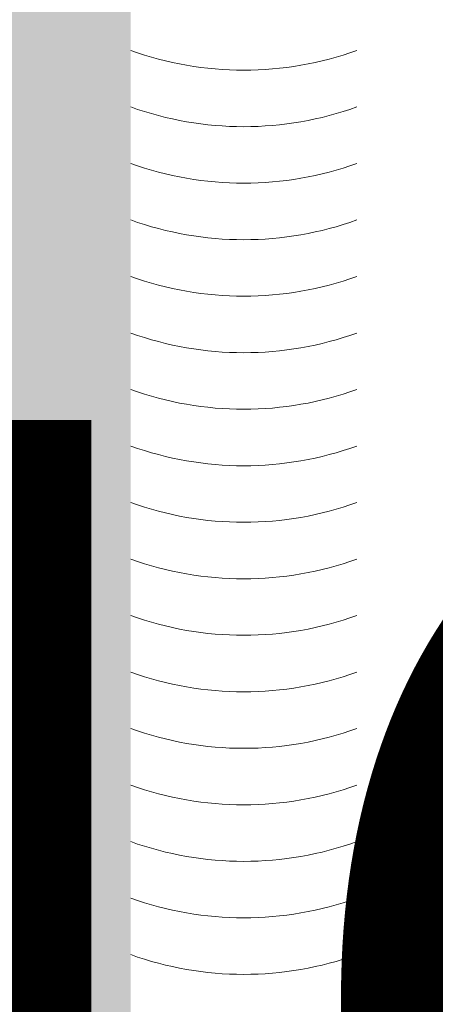
# Model space of a CAD drawing. Units: inches. Extents: x 844 to 2234, y 346 to 1084.
# Tile 85 of 93: x 2010.294 to 2012.46, y 701.365 to 706.497. Entities that reach past the tile are written whole.
import ezdxf

# ---------------------------------------------------------------- set-up
doc = ezdxf.new("R2010")
doc.units = ezdxf.units.IN
doc.header["$MEASUREMENT"] = 0
for name, color, linetype, lineweight in [('A-ANNO-DIMS', 2, 'Continuous', 18), ('furniture', 8, 'Continuous', 18), ('RA-AP-01$0$INT', 35, 'Continuous', 5)]:
    doc.layers.add(name, color=color, linetype=linetype, lineweight=lineweight)
doc.layers.add('RA-AP-01$0$FURN', color=3, linetype='Continuous')
doc.styles.get("Standard").update_dxf_attribs({"font": 'arial.ttf'})
doc.dimstyles.get("Standard").update_dxf_attribs({"dimtxt": 6, "dimasz": 3, "dimexe": 0.18, "dimexo": 0.0625, "dimgap": 0.09, "dimtad": 0, "dimtih": 1, "dimtoh": 1, "dimdec": 1, "dimzin": 0, "dimdsep": 46, "dimlunit": 3, "dimtxsty": 'Standard', "dimblk": 'ARCHTICK', "dimcen": 0.09, "dimadec": 0, "dimazin": 0, "dimtfac": 1, "dimtdec": 1, "dimtofl": 0, "dimtmove": 0, "dimatfit": 3, "dimfxl": 1, "dimtolj": 1, "dimtzin": 0, "dimarcsym": 0})

# ---------------------------------------------------------------- blocks, each defined once
blk = doc.blocks.new('A$C18D01794')
at = {"layer": 'RA-AP-01$0$INT'}
h = blk.add_hatch(color=256, dxfattribs=at)
h.paths.add_polyline_path([(4.355206456958071, -6.156712009588037), (4.355206456958071, -8.056712009588038), (5.455206456958072, -8.056712009588038), (5.455206456958072, -6.156712009588037)])
h.paths.add_polyline_path([(4.405206456958072, -8.006712009588039), (4.405206456958072, -6.206712009588038), (5.405206456958072, -6.206712009588038), (5.405206456958072, -8.006712009588039)], flags=16)
for centre in [(4.309006456955269, -7.255364458282008), (4.309006456955269, -7.278464458280756), (4.309006456953677, -7.301564458285417), (4.309006456954814, -7.324664458284166), (4.309006456954814, -7.347764458279732), (4.309006456953222, -7.37086445828462), (4.309006456955951, -7.393964458283369), (4.309006456955951, -7.417064458282117), (4.309006456954359, -7.440164458286778), (4.309006456955496, -7.463264458285527), (4.309006456955496, -7.486364458281093), (4.309006456953905, -7.509464458285981), (4.309006456952086, -7.532564458284502), (4.309006456955041, -7.555664458280295), (4.309006456954814, -7.578764458284956), (4.309006456953222, -7.601864458283705), (4.309006456951631, -7.624964458285409)]:
    blk.add_arc(centre, 0.136414042854523, 70.20384312815696, 109.7961568705686, dxfattribs=at)
blk = doc.blocks.new('A$C5D2F253E')
at = {"layer": 'RA-AP-01$0$FURN', "xscale": -0.7999999999883585, "yscale": 0.7999999999883585, "zscale": 0.8, "rotation": 90}
blk.add_blockref('A$C18D01794', (-5.687757199772477, 4.75791982714071), dxfattribs=at)
blk = doc.blocks.new('_ArchTick')
at = {"color": 0, "linetype": 'ByBlock', "const_width": 0.15}
blk.add_lwpolyline([(-0.5, -0.5), (0.5, 0.5)], dxfattribs=at)
blk = doc.blocks.new('*D121')
at = {"layer": 'A-ANNO-DIMS', "color": 0, "lineweight": -2, "transparency": 16777216}
for p, q in [((2030.271987351997, 734.262611118704), (2040.245275089302, 734.262611118704)), ((2040.065275089302, 734.262611118704), (2040.065275089302, 704.6043509484256)), ((2040.065275089302, 668.557359536674), (2040.065275089302, 698.2156197069523)), ((2030.271987351997, 668.557359536674), (2040.245275089302, 668.557359536674))]:
    blk.add_line(p, q, dxfattribs=at)
at = {"layer": 'Defpoints', "color": 0, "transparency": 16777216}
for p in [(2030.209487351997, 734.262611118704), (2040.065275089302, 734.262611118704), (2030.209487351997, 668.557359536674)]:
    blk.add_point(p, dxfattribs=at)
at = {"layer": 'A-ANNO-DIMS', "color": 0, "lineweight": -2, "transparency": 16777216, "xscale": 3, "yscale": 3, "zscale": 3}
for p, rotation in [((2040.065275089302, 734.262611118704), 90), ((2040.065275089302, 668.557359536674), 270)]:
    blk.add_blockref('_ArchTick', p, dxfattribs=dict(at, rotation=rotation))
at = {"layer": 'A-ANNO-DIMS', "color": 0, "transparency": 16777216, "insert": (2040.065275089302, 701.4099853276883), "char_height": 6, "attachment_point": 5}
blk.add_mtext('\\A1;LOUNGE SET 5\'-5 1/2" TYP.', dxfattribs=at)

msp = doc.modelspace()

# ---------------------------------------------------------------- block references
at = {"layer": 'furniture', "xscale": -15.94108302203742, "yscale": 15.94108302203742, "zscale": 15.94108302203742, "rotation": 270}
msp.add_blockref('A$C5D2F253E', (1990.567271852805, 701.4028671565849), dxfattribs=at)

# ---------------------------------------------------------------- dimensions: what is measured, and where the dimension line sits
at = {"layer": 'A-ANNO-DIMS'}
dim = msp.add_linear_dim(base=(2040.065275089302, 734.262611118704), p1=(2030.209487351996, 668.5573595366737), p2=(2030.209487351996, 734.2626111187037), angle=90, text='LOUNGE SET <> TYP.', dimstyle='Standard', override={"dimdec": 1, "dimlfac": 1, "dimrnd": 0, "dimzin": 1, "dimdsep": 46, "dimlunit": 4, "dimfrac": 2}, dxfattribs=at)
dim.commit()
dim.dimension.update_dxf_attribs({"geometry": '*D121', "text_midpoint": (2040.065275089302, 701.4099853276883)})

doc.saveas('drawing.dxf')
